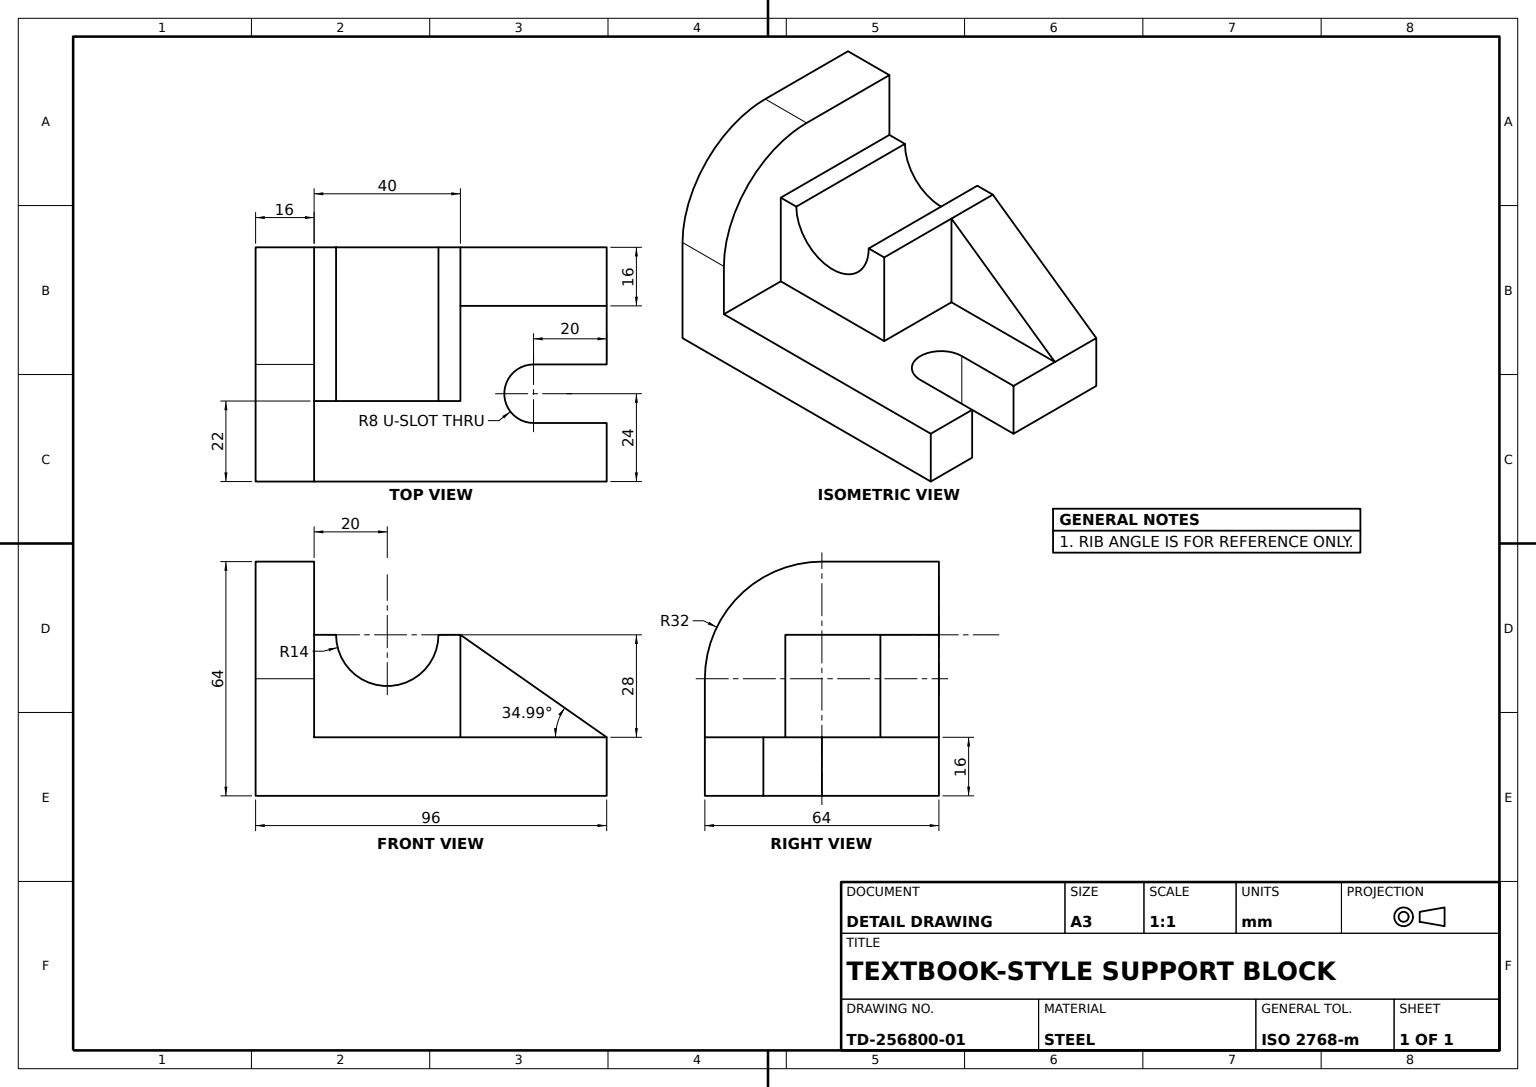
from build123d import *

# Parameters (mm, degrees)
BASE_PLATE_SKETCH_W         = 96
BASE_PLATE_SKETCH_H         = 64
BASE_PLATE_96X64X16_DEPTH   = 16
U_SLOT_DEPTH                = 16
UPRIGHT_R32_DEPTH           = 16
CRADLE_BLOCK_SKETCH_W       = 40
CRADLE_BLOCK_SKETCH_H       = 42
CRADLE_BLOCK_40X22X28_DEPTH = 28
CRADLE_BORE_SKETCH_R        = 14
CRADLE_BORE_28_DEPTH        = 123.784363825
GUSSET_RIB_DEPTH            = 16


with BuildPart() as part:
    # Base Plate Sketch → Base Plate 96x64x16 (new body)
    with BuildSketch(Plane(origin=(0, 0, 0), x_dir=(1, 0, 0), z_dir=(0, 1, 0))):
        with Locations((48, 32)):
            Rectangle(BASE_PLATE_SKETCH_W, BASE_PLATE_SKETCH_H)
    extrude(amount=BASE_PLATE_96X64X16_DEPTH)

    # U-Slot Sketch → U-Slot (cut)
    with BuildSketch(Plane(origin=(0, 16, 0), x_dir=(1, 0, 0), z_dir=(0, 1, 0))):
        with BuildLine():
            Line((96, 16), (76, 16))
            ThreePointArc((76, 16), (68, 24), (76, 32))
            Line((76, 32), (96, 32))
            ThreePointArc((96, 32), (104, 24), (96, 16))
        make_face()
    extrude(amount=-U_SLOT_DEPTH, mode=Mode.SUBTRACT)

    # Upright Sketch → Upright R32 (add)
    with BuildSketch(Plane.ZY):
        with BuildLine():
            Line((-64, 0), (0, 0))
            Line((0, 0), (0, 32))
            ThreePointArc((0, 32), (-9.372583002, 54.627416998), (-32, 64))
            Line((-32, 64), (-64, 64))
            Line((-64, 64), (-64, 0))
        make_face()
    extrude(amount=-UPRIGHT_R32_DEPTH)

    # Cradle Block Sketch → Cradle Block 40x22x28 (add)
    with BuildSketch(Plane(origin=(0, 16, 0), x_dir=(1, 0, 0), z_dir=(0, 1, 0))):
        with Locations((36, 43)):
            Rectangle(CRADLE_BLOCK_SKETCH_W, CRADLE_BLOCK_SKETCH_H)
    extrude(amount=CRADLE_BLOCK_40X22X28_DEPTH)

    # Cradle Bore Sketch → Cradle Bore Ø28 (cut, through all)
    with BuildSketch(Plane.XY.offset(-22)):
        with Locations((36, 44)):
            Circle(CRADLE_BORE_SKETCH_R)
    extrude(amount=-CRADLE_BORE_28_DEPTH, mode=Mode.SUBTRACT)

    # Gusset Rib Sketch → Gusset Rib (add)
    with BuildSketch(Plane(origin=(0, 0, -64), x_dir=(-1, 0, 0), z_dir=(0, 0, -1))):
        Polygon((-56, 44), (-56, 16), (-96, 16), align=None)
    extrude(amount=-GUSSET_RIB_DEPTH)


solid = part.part
